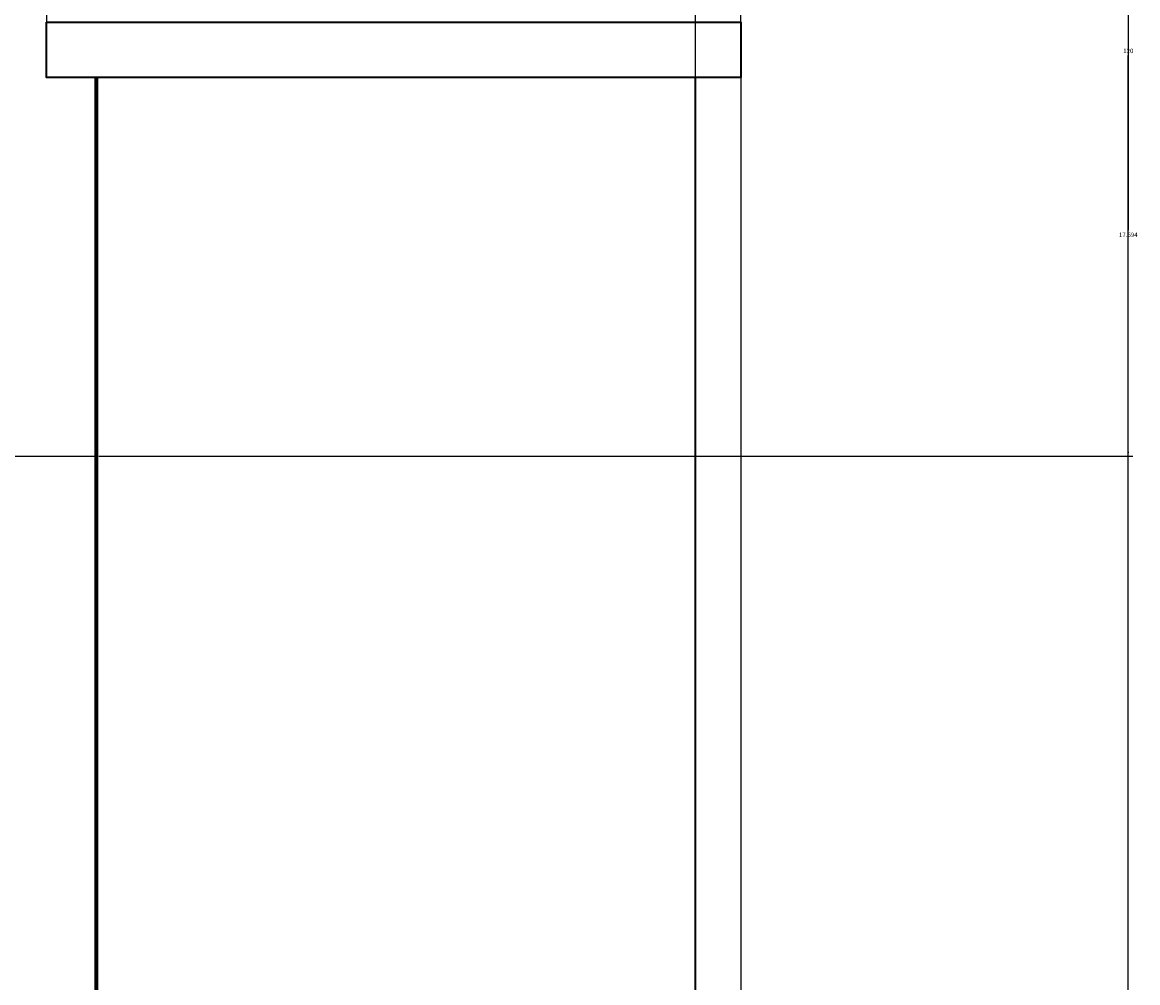
# Model space of a CAD drawing. Units: inches. Extents: x -6 to 289, y -8 to 323.
# Tile 36 of 107: x 244 to 289, y 30 to 68. Entities that reach past the tile are written whole.
import ezdxf

# ---------------------------------------------------------------- set-up
doc = ezdxf.new("R2010")
doc.units = ezdxf.units.IN
doc.header["$MEASUREMENT"] = 0
for name, color, linetype, lineweight in [('A-ANNO-DIMS', 2, 'Continuous', 18), ('A-DOOR', 3, 'Continuous', 25), ('A-ELEV', 7, 'Continuous', 35)]:
    doc.layers.add(name, color=color, linetype=linetype, lineweight=lineweight)
doc.styles.get("Standard").update_dxf_attribs({"font": 'arial.ttf'})
doc.dimstyles.get("Standard").update_dxf_attribs({"dimtxt": 0.18, "dimasz": 0.18, "dimexe": 0.18, "dimexo": 0.0625, "dimgap": 0.09, "dimtad": 0, "dimtih": 1, "dimtoh": 1, "dimdec": 4, "dimzin": 0, "dimdsep": 46, "dimtxsty": 'Standard', "dimcen": 0.09, "dimadec": 0, "dimazin": 0, "dimtfac": 1, "dimtdec": 4, "dimtofl": 0, "dimtmove": 0, "dimatfit": 3, "dimfxl": 1, "dimtolj": 1, "dimtzin": 0, "dimarcsym": 0})

# ---------------------------------------------------------------- blocks, each defined once
blk = doc.blocks.new('*D15')
at = {"layer": 'A-ANNO-DIMS', "color": 0, "lineweight": -2, "transparency": 16777216}
for p, q in [((247.164, 162.411), (247.164, 322.969)), ((271.164, 7.351), (271.164, 322.969)), ((247.344, 322.789), (258.944, 322.789)), ((270.984, 322.789), (259.384, 322.789))]:
    blk.add_line(p, q, dxfattribs=at)
at = {"layer": 'A-ANNO-DIMS', "color": 0, "transparency": 16777216}
for points in [[(247.344, 322.819), (247.344, 322.759), (247.164, 322.789)], [(270.984, 322.819), (270.984, 322.759), (271.164, 322.789)]]:
    blk.add_solid(points, dxfattribs=at)
at = {"layer": 'Defpoints', "color": 0, "transparency": 16777216}
for p in [(271.164, 322.789), (247.164, 162.348), (271.164, 7.289)]:
    blk.add_point(p, dxfattribs=at)
at = {"layer": 'A-ANNO-DIMS', "color": 0, "transparency": 16777216, "insert": (259.164, 322.789), "char_height": 0.18, "attachment_point": 5}
blk.add_mtext('\\A1;24', dxfattribs=at)
blk = doc.blocks.new('*D16')
at = {"layer": 'A-ANNO-DIMS', "color": 0, "lineweight": -2, "transparency": 16777216}
for p, q in [((9.943, 68.37), (9.943, -8.391)), ((272.973, 68.37), (272.973, -8.391)), ((10.123, -8.211), (140.993, -8.211)), ((272.793, -8.211), (141.923, -8.211))]:
    blk.add_line(p, q, dxfattribs=at)
at = {"layer": 'A-ANNO-DIMS', "color": 0, "transparency": 16777216}
for points in [[(10.123, -8.181), (10.123, -8.241), (9.943, -8.211)], [(272.793, -8.181), (272.793, -8.241), (272.973, -8.211)]]:
    blk.add_solid(points, dxfattribs=at)
at = {"layer": 'Defpoints', "color": 0, "transparency": 16777216}
for p in [(9.943, 68.432), (272.973, 68.432), (272.973, -8.211)]:
    blk.add_point(p, dxfattribs=at)
at = {"layer": 'A-ANNO-DIMS', "color": 0, "transparency": 16777216, "insert": (141.458, -8.211), "char_height": 0.18, "attachment_point": 5}
blk.add_mtext('\\A1;263.03', dxfattribs=at)
blk = doc.blocks.new('*D23')
at = {"layer": 'A-ANNO-DIMS', "color": 0, "lineweight": -2, "transparency": 16777216}
for p, q in [((259.226, 127.289), (288.653, 127.289)), ((288.473, 127.109), (288.473, 67.471)), ((288.473, 7.469), (288.473, 67.107)), ((271.226, 7.289), (288.653, 7.289))]:
    blk.add_line(p, q, dxfattribs=at)
at = {"layer": 'A-ANNO-DIMS', "color": 0, "transparency": 16777216}
for points in [[(288.443, 127.109), (288.503, 127.109), (288.473, 127.289)], [(288.443, 7.469), (288.503, 7.469), (288.473, 7.289)]]:
    blk.add_solid(points, dxfattribs=at)
at = {"layer": 'Defpoints', "color": 0, "transparency": 16777216}
for p in [(259.164, 127.289), (288.473, 127.289), (271.164, 7.289)]:
    blk.add_point(p, dxfattribs=at)
at = {"layer": 'A-ANNO-DIMS', "color": 0, "transparency": 16777216, "insert": (288.473, 67.289), "char_height": 0.18, "attachment_point": 5}
blk.add_mtext('\\A1;120', dxfattribs=at)
blk = doc.blocks.new('*D81')
at = {"layer": 'A-ANNO-DIMS', "color": 0, "lineweight": -2, "transparency": 16777216}
for p, q in [((230.292, 68.842), (230.292, 322.969)), ((245.215, 66.286), (245.215, 322.969)), ((230.472, 322.789), (237.298, 322.789)), ((245.035, 322.789), (238.208, 322.789))]:
    blk.add_line(p, q, dxfattribs=at)
at = {"layer": 'A-ANNO-DIMS', "color": 0, "transparency": 16777216}
for points in [[(230.472, 322.819), (230.472, 322.759), (230.292, 322.789)], [(245.035, 322.819), (245.035, 322.759), (245.215, 322.789)]]:
    blk.add_solid(points, dxfattribs=at)
at = {"layer": 'Defpoints', "color": 0, "transparency": 16777216}
for p in [(245.215, 322.789), (230.292, 68.779), (245.215, 66.224)]:
    blk.add_point(p, dxfattribs=at)
at = {"layer": 'A-ANNO-DIMS', "color": 0, "transparency": 16777216, "insert": (237.753, 322.789), "char_height": 0.18, "attachment_point": 5}
blk.add_mtext('\\A1;14.923', dxfattribs=at)
blk = doc.blocks.new('*D82')
at = {"layer": 'A-ANNO-DIMS', "color": 0, "lineweight": -2, "transparency": 16777216}
for p, q in [((245.215, 66.286), (245.215, 322.969)), ((272.973, 66.286), (272.973, 322.969)), ((245.395, 322.789), (258.699, 322.789)), ((272.793, 322.789), (259.489, 322.789))]:
    blk.add_line(p, q, dxfattribs=at)
at = {"layer": 'A-ANNO-DIMS', "color": 0, "transparency": 16777216}
for points in [[(245.395, 322.819), (245.395, 322.759), (245.215, 322.789)], [(272.793, 322.819), (272.793, 322.759), (272.973, 322.789)]]:
    blk.add_solid(points, dxfattribs=at)
at = {"layer": 'Defpoints', "color": 0, "transparency": 16777216}
for p in [(272.973, 322.789), (245.215, 66.224), (272.973, 66.224)]:
    blk.add_point(p, dxfattribs=at)
at = {"layer": 'A-ANNO-DIMS', "color": 0, "transparency": 16777216, "insert": (259.094, 322.789), "char_height": 0.18, "attachment_point": 5}
blk.add_mtext('\\A1;27.76', dxfattribs=at)
blk = doc.blocks.new('*D90')
at = {"layer": 'A-ANNO-DIMS', "color": 0, "lineweight": -2, "transparency": 16777216}
for p, q in [((230.354, 68.779), (288.653, 68.779)), ((288.473, 68.599), (288.473, 60.114)), ((288.473, 51.265), (288.473, 59.75)), ((247.303, 51.085), (288.653, 51.085))]:
    blk.add_line(p, q, dxfattribs=at)
at = {"layer": 'A-ANNO-DIMS', "color": 0, "transparency": 16777216}
for points in [[(288.443, 68.599), (288.503, 68.599), (288.473, 68.779)], [(288.443, 51.265), (288.503, 51.265), (288.473, 51.085)]]:
    blk.add_solid(points, dxfattribs=at)
at = {"layer": 'Defpoints', "color": 0, "transparency": 16777216}
for p in [(230.292, 68.779), (288.473, 68.779), (247.241, 51.085)]:
    blk.add_point(p, dxfattribs=at)
at = {"layer": 'A-ANNO-DIMS', "color": 0, "transparency": 16777216, "insert": (288.473, 59.932), "char_height": 0.18, "attachment_point": 5}
blk.add_mtext('\\A1;17.694', dxfattribs=at)

msp = doc.modelspace()

# ---------------------------------------------------------------- linework, layer by layer
at = {"layer": 'A-DOOR'}
msp.add_lwpolyline([(121.008, 51.0851), (247.2408, 51.0851), (247.2408, 7.2888), (121.008, 7.2888)], close=True, dxfattribs=at)
at = {"layer": 'A-ELEV'}
for p, q in [((247.1638, 7.2888), (247.1638, 66.2238)), ((247.2408, 66.2238), (247.2408, 7.2888)), ((271.1638, 7.2888), (271.1638, 66.2238))]:
    msp.add_line(p, q, dxfattribs=at)
msp.add_lwpolyline([(245.2146, 68.4322), (272.9733, 68.4322), (272.9733, 66.2238), (245.2146, 66.2238)], close=True, dxfattribs=at)

# ---------------------------------------------------------------- dimensions: what is measured, and where the dimension line sits
at = {"layer": 'A-ANNO-DIMS'}
for base, p1, p2, override, picture, middle in [((245.2146, 322.7888), (230.2918, 68.7795), (245.2146, 66.2238), {"dimdec": 3, "dimlfac": 1, "dimrnd": 0, "dimzin": 0, "dimdsep": 46, "dimlunit": 2}, '*D81', (237.7532, 322.7888)), ((272.9733, 322.7888), (245.2146, 66.2238), (272.9733, 66.2238), {"dimdec": 2, "dimlfac": 1, "dimrnd": 0, "dimzin": 0, "dimdsep": 46, "dimlunit": 2}, '*D82', (259.0939, 322.7888)), ((271.1638, 322.7888), (247.1638, 162.3484), (271.1638, 7.2888), {"dimdec": 0, "dimlfac": 1, "dimrnd": 0, "dimzin": 0, "dimdsep": 46, "dimlunit": 2}, '*D15', (259.1638, 322.7888)), ((272.9733, -8.2112), (9.943, 68.4322), (272.9733, 68.4322), {"dimdec": 2, "dimlfac": 1, "dimrnd": 0, "dimzin": 0, "dimdsep": 46, "dimlunit": 2}, '*D16', (141.4581, -8.2112))]:
    dim = msp.add_linear_dim(base=base, p1=p1, p2=p2, dimstyle='Standard', override=override, dxfattribs=at)
    dim.commit()
    dim.dimension.update_dxf_attribs({"geometry": picture, "text_midpoint": middle})
for base, p1, p2, override, picture, middle in [((288.4733, 127.2888), (271.1638, 7.2888), (259.1638, 127.2888), {"dimdec": 0, "dimlfac": 1, "dimrnd": 0, "dimzin": 0, "dimdsep": 46, "dimlunit": 2}, '*D23', (288.4733, 67.2888)), ((288.4733, 68.7795), (247.2408, 51.0851), (230.2918, 68.7795), {"dimdec": 3, "dimlfac": 1, "dimrnd": 0, "dimzin": 0, "dimdsep": 46, "dimlunit": 2}, '*D90', (288.4733, 59.9323))]:
    dim = msp.add_linear_dim(base=base, p1=p1, p2=p2, angle=90, dimstyle='Standard', override=override, dxfattribs=at)
    dim.commit()
    dim.dimension.update_dxf_attribs({"geometry": picture, "text_midpoint": middle})

doc.saveas('drawing.dxf')
